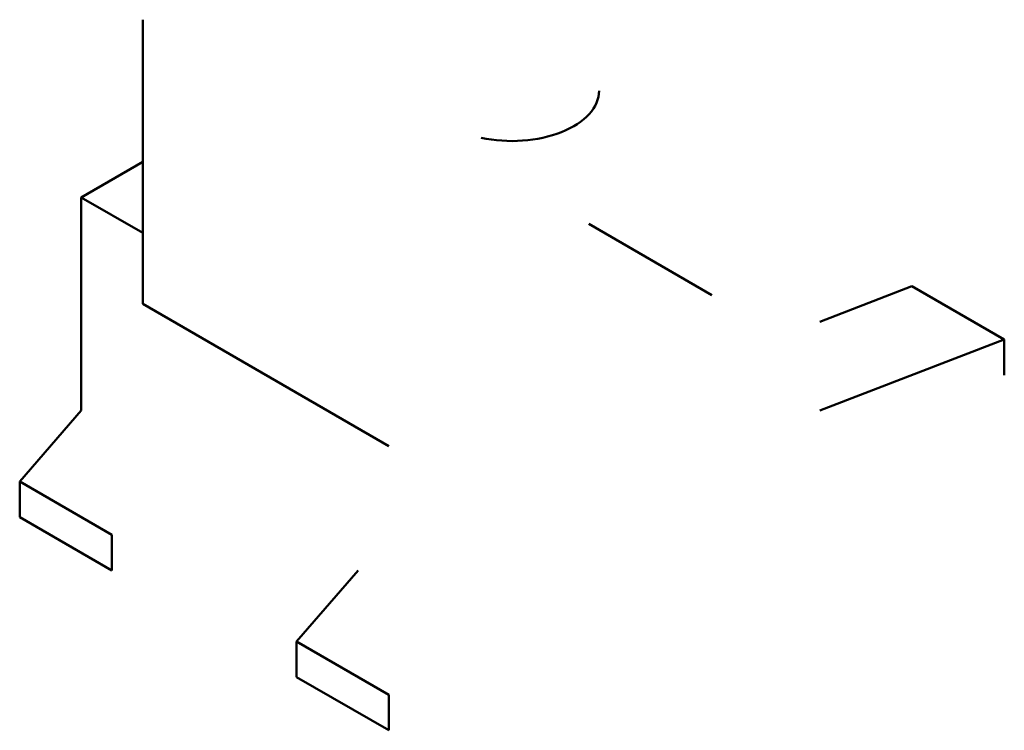
# Model space of a CAD drawing. Units: inches. Extents: x 595 to 18402, y 316 to 10662.
# Tile 2 of 2: x 14882 to 18402, y 8122 to 10662. Entities that reach past the tile are written whole.
import ezdxf

# ---------------------------------------------------------------- set-up
doc = ezdxf.new("R2010")
doc.units = ezdxf.units.IN
doc.header["$MEASUREMENT"] = 0
doc.layers.add('M-OUTL', color=7, linetype='Continuous', lineweight=50)

msp = doc.modelspace()

# ---------------------------------------------------------------- linework, layer by layer
at = {"layer": 'M-OUTL'}
for p, q in [((15322.2, 9646), (15322.2, 10662)), ((15102.2, 10027), (15322.2, 10154)), ((15102.2, 9265), (15102.2, 10027)), ((15322.2, 9900), (15102.2, 10027)), ((17356.9, 9677.8), (16917, 9931.8)), ((18071.8, 9709.5), (17741.9, 9582.5)), ((18401.8, 9519), (18071.8, 9709.5)), ((16202.1, 9138), (15322.2, 9646)), ((18401.8, 9519), (17741.9, 9265)), ((18401.8, 9392), (18401.8, 9519)), ((15102.2, 9265), (14882.3, 9011)), ((15212.2, 8820.5), (14882.3, 9011)), ((14882.3, 9011), (14882.3, 8884)), ((15212.2, 8693.5), (14882.3, 8884)), ((15212.2, 8820.5), (15212.2, 8693.5)), ((16092.1, 8693.5), (15872.1, 8439.5)), ((15872.1, 8439.5), (15872.1, 8312.5)), ((16202.1, 8249), (15872.1, 8439.5)), ((16202.1, 8122), (15872.1, 8312.5)), ((16202.1, 8249), (16202.1, 8122))]:
    msp.add_line(p, q, dxfattribs=at)
msp.add_ellipse((16642, 10408), major_axis=(311.1, 0), ratio=0.57735, start_param=4.351022, end_param=6.283185, dxfattribs=at)

doc.saveas('drawing.dxf')
